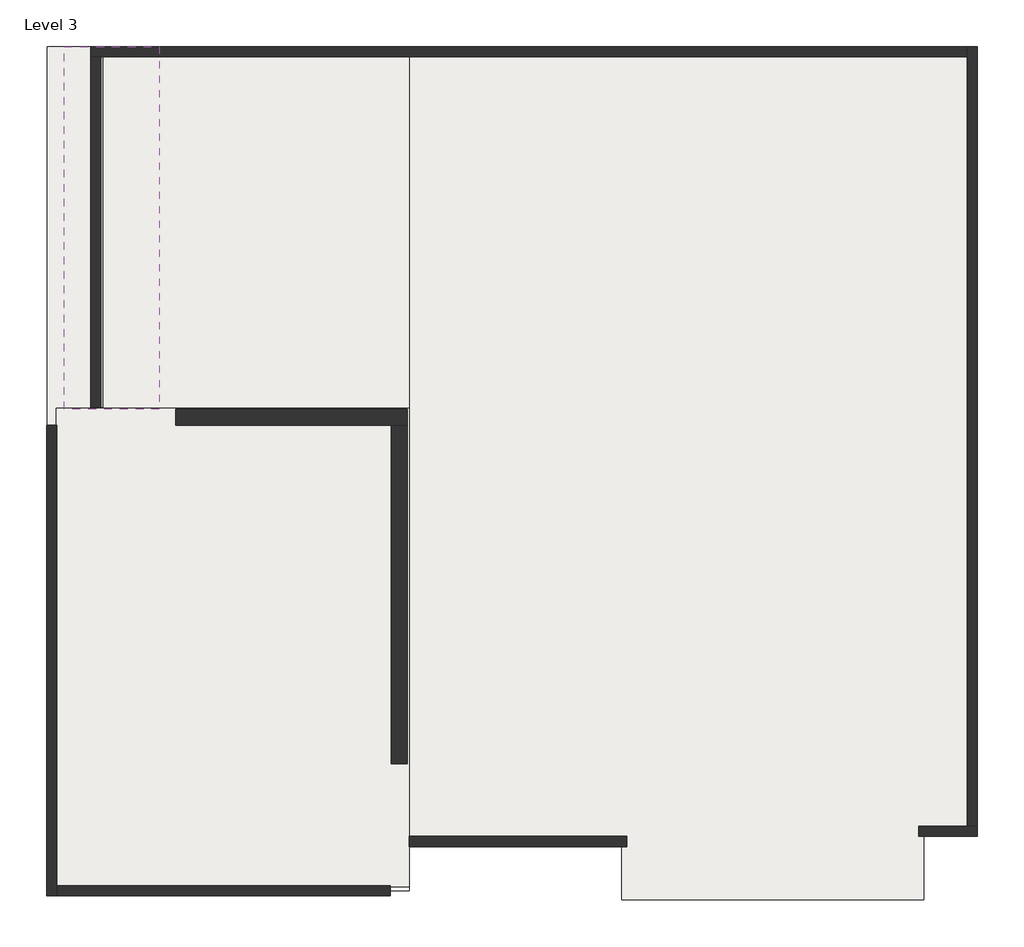
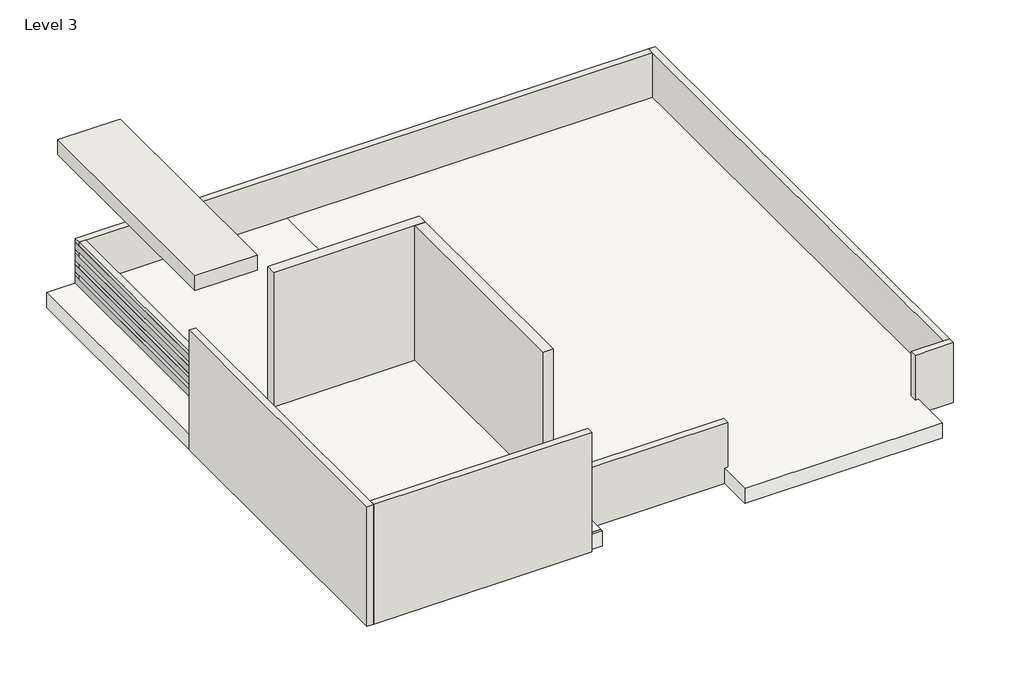
# One storey, incomplete: 10 walls, 4 proxies, 3 roofs.
"""IFC4 building model written with IfcOpenShell, lengths in millimetres."""

from ifc_helpers import new_model, si_unit, frame, origin, place, context, project, spatial, polyline, outline, extrude, faceted_brep, transform, mapped, element, save
from components import walls_6_walls_6_3012a6d8

model = new_model("IFC4")

# Units and contexts
model_context = context("Model", 3, world=origin())
ifc_project = project(units=[si_unit("LENGTHUNIT", "METRE", prefix="MILLI")], contexts=[model_context])

# Site, building, storey
site = spatial("IfcSite", under=ifc_project)
building = spatial("IfcBuilding", under=site)
storey = spatial("IfcBuildingStorey", under=building, Name="Level 3", Elevation=7315.2)

# Proxies
placement = place(None, origin())
element("IfcBuildingElementProxy", 1, Name="Reveal", ObjectType="Reveal", at=placement, inside=storey, context=model_context, shape_type="SweptSolid", body=[
    extrude(outline(polyline([(-11786.2932708, 11358.0609482), (-11633.8932708, 11358.0609482), (-11633.8932708, 6811.4609482), (-11786.2932708, 6811.4609482), (-11786.2932708, 11358.0609482)])), frame((0.0, 0.0, 8309.1450158), z_axis=(0.0, 0.0, 1.0), x_axis=(1.0, 0.0, 0.0)), (0.0, 0.0, 1.0), 152.4),
])
element("IfcBuildingElementProxy", 2, Name="Reveal", ObjectType="Reveal", at=placement, inside=storey, context=model_context, shape_type="SweptSolid", body=[
    extrude(outline(polyline([(-11786.2932708, 11358.0609482), (-11633.8932708, 11358.0609482), (-11633.8932708, 6811.4609482), (-11786.2932708, 6811.4609482), (-11786.2932708, 11358.0609482)])), frame((0.0, 0.0, 8080.5450158), z_axis=(0.0, 0.0, 1.0), x_axis=(1.0, 0.0, 0.0)), (0.0, 0.0, 1.0), 152.4),
])
element("IfcBuildingElementProxy", 3, Name="Reveal", ObjectType="Reveal", at=placement, inside=storey, context=model_context, shape_type="SweptSolid", body=[
    extrude(outline(polyline([(-11786.2932708, 11358.0609482), (-11633.8932708, 11358.0609482), (-11633.8932708, 6811.4609482), (-11786.2932708, 6811.4609482), (-11786.2932708, 11358.0609482)])), frame((0.0, 0.0, 7851.9450158), z_axis=(0.0, 0.0, 1.0), x_axis=(1.0, 0.0, 0.0)), (0.0, 0.0, 1.0), 152.4),
])
element("IfcBuildingElementProxy", 4, Name="Reveal", ObjectType="Reveal", at=placement, inside=storey, context=model_context, shape_type="SweptSolid", body=[
    extrude(outline(polyline([(-11786.2932708, 11358.0609482), (-11633.8932708, 11358.0609482), (-11633.8932708, 6811.4609482), (-11786.2932708, 6811.4609482), (-11786.2932708, 11358.0609482)])), frame((0.0, 0.0, 7620.0), z_axis=(0.0, 0.0, 1.0), x_axis=(1.0, 0.0, 0.0)), (0.0, 0.0, 1.0), 152.4),
])

# Roofs
element("IfcRoof", 5, ObjectType="Generic - 12\"", at=placement, inside=storey, context=model_context, shape_type="SweptSolid", body=[
    extrude(outline(polyline([(-11786.2932708, 11358.0609482), (-610.2932708, 11358.0609482), (-610.2932708, 1401.2609482), (-1286.2833771, 1401.2609482), (-1286.2833771, 600.2635335), (-5096.2833771, 600.2635335), (-5096.2833771, 1401.2609482), (-7773.0932708, 1401.2609482), (-7773.0932708, 1071.0609482), (-12218.0932708, 1071.0609482), (-12218.0932708, 6786.0609482), (-11786.2932708, 6786.0609482), (-11786.2932708, 11358.0609482)])), frame((0.0, 0.0, 7315.2), z_axis=(0.0, 0.0, 1.0), x_axis=(1.0, 0.0, 0.0)), (0.0, 0.0, 1.0), 304.8),
])
element("IfcRoof", 6, ObjectType="Generic - 12\"", at=placement, inside=storey, context=model_context, shape_type="SweptSolid", body=[
    extrude(outline(polyline([(-12338.7432708, 11358.0609482), (-7773.0932708, 11358.0609482), (-7773.0932708, 714.9399767), (-12338.7432708, 714.9399767), (-12338.7432708, 11358.0609482)])), frame((0.0, 0.0, 7315.2), z_axis=(0.0, 0.0, 1.0), x_axis=(1.0, 0.0, 0.0)), (0.0, 0.0, 1.0), 304.8),
])
element("IfcRoof", 7, ObjectType="Generic - 12\"", at=placement, inside=storey, context=model_context, shape_type="SweptSolid", body=[
    extrude(outline(polyline([(-7773.0932708, 765.7399767), (-12223.0431118, 765.7399767), (-12223.0431118, 6798.7609482), (-7773.0932708, 6798.7609482), (-7773.0932708, 765.7399767)])), frame((0.0, 0.0, 7315.2), z_axis=(0.0, 0.0, 1.0), x_axis=(1.0, 0.0, 0.0)), (0.0, 0.0, 1.0), 304.8),
])

# Walls
element("IfcWall", 8, ObjectType="Generic - 5\"", at=placement, inside=storey, context=model_context, shape_type="Brep", body=[
    faceted_brep([(-12345.0932708, 6582.8609482, 7315.2), (-12345.0932708, 651.9609482, 7315.2), (-12345.0932708, 651.9609482, 9753.6), (-12345.0932708, 6582.8609482, 9753.6), (-12218.0932708, 6582.8609482, 7315.2), (-12218.0932708, 6582.8609482, 9753.6), (-12218.0932708, 778.9609482, 9753.6), (-12218.0932708, 651.9609482, 9753.6), (-12218.0932708, 651.9609482, 7315.2), (-12218.0932708, 778.9609482, 7315.2)], [[[0, 1, 2, 3]], [[4, 5, 6, 7, 8, 9]], [[1, 0, 4, 9, 8]], [[3, 2, 7, 6, 5]], [[0, 3, 5, 4]], [[2, 1, 8, 7]]]),
])
element("IfcWall", 9, ObjectType="Generic - 5\"", at=placement, inside=storey, context=model_context, shape_type="SweptSolid", body=[
    extrude(outline(polyline([(-8014.3932708, 651.9609482), (-12218.0932708, 651.9609482), (-12218.0932708, 778.9609482), (-8014.3932708, 778.9609482), (-8014.3932708, 651.9609482)])), frame((0.0, 0.0, 7315.2), z_axis=(0.0, 0.0, 1.0), x_axis=(1.0, 0.0, 0.0)), (0.0, 0.0, 1.0), 2438.4),
])
element("IfcWall", 10, ObjectType="Generic - 5\"", at=placement, inside=storey, context=model_context, shape_type="Brep", body=[
    faceted_brep([(-1349.7833771, 1401.2609482, 7315.2), (-610.2932708, 1401.2609482, 7315.2), (-610.2932708, 1401.2609482, 8534.4), (-1349.7833771, 1401.2609482, 8534.4), (-1349.7833771, 1528.2609482, 7315.2), (-1349.7833771, 1528.2609482, 8534.4), (-737.2932708, 1528.2609482, 8534.4), (-610.2932708, 1528.2609482, 8534.4), (-610.2932708, 1528.2609482, 7315.2), (-737.2932708, 1528.2609482, 7315.2)], [[[0, 1, 2, 3]], [[4, 5, 6, 7, 8, 9]], [[1, 0, 4, 9, 8]], [[3, 2, 7, 6, 5]], [[0, 3, 5, 4]], [[2, 1, 8, 7]]]),
])
element("IfcWall", 11, ObjectType="Generic - 5\"", at=placement, inside=storey, context=model_context, shape_type="SweptSolid", body=[
    extrude(outline(polyline([(-7773.0932708, 1401.2609482), (-5032.7833771, 1401.2609482), (-5032.7833771, 1274.2609482), (-7773.0932708, 1274.2609482), (-7773.0932708, 1401.2609482)])), frame((0.0, 0.0, 7315.2), z_axis=(0.0, 0.0, 1.0), x_axis=(1.0, 0.0, 0.0)), (0.0, 0.0, 1.0), 1219.2),
])
element("IfcWall", 12, ObjectType="Generic - 5\"", at=placement, inside=storey, context=model_context, shape_type="Brep", body=[
    faceted_brep([(-610.2932708, 1528.2609482, 7315.2), (-610.2932708, 11358.0609482, 7315.2), (-610.2932708, 11358.0609482, 8534.4), (-610.2932708, 1528.2609482, 8534.4), (-737.2932708, 1528.2609482, 7315.2), (-737.2932708, 1528.2609482, 8534.4), (-737.2932708, 11231.0609482, 8534.4), (-737.2932708, 11358.0609482, 8534.4), (-737.2932708, 11358.0609482, 7315.2), (-737.2932708, 11231.0609482, 7315.2)], [[[0, 1, 2, 3]], [[4, 5, 6, 7, 8, 9]], [[1, 0, 4, 9, 8]], [[3, 2, 7, 6, 5]], [[0, 3, 5, 4]], [[2, 1, 8, 7]]]),
])
element("IfcWall", 13, ObjectType="Generic - 5\"", at=placement, inside=storey, context=model_context, shape_type="Brep", body=[
    faceted_brep([(-737.2932708, 11358.0609482, 7315.2), (-11786.2932708, 11358.0609482, 7315.2), (-11786.2932708, 11358.0609482, 7620.0), (-11633.8932708, 11358.0609482, 7620.0), (-11633.8932708, 11358.0609482, 7772.4), (-11786.2932708, 11358.0609482, 7772.4), (-11786.2932708, 11358.0609482, 7851.9450158), (-11633.8932708, 11358.0609482, 7851.9450158), (-11633.8932708, 11358.0609482, 8004.3450158), (-11786.2932708, 11358.0609482, 8004.3450158), (-11786.2932708, 11358.0609482, 8080.5450158), (-11633.8932708, 11358.0609482, 8080.5450158), (-11633.8932708, 11358.0609482, 8232.9450158), (-11786.2932708, 11358.0609482, 8232.9450158), (-11786.2932708, 11358.0609482, 8309.1450158), (-11633.8932708, 11358.0609482, 8309.1450158), (-11633.8932708, 11358.0609482, 8461.5450158), (-11786.2932708, 11358.0609482, 8461.5450158), (-11786.2932708, 11358.0609482, 8534.4), (-737.2932708, 11358.0609482, 8534.4), (-11786.2932708, 11231.0609482, 7315.2), (-737.2932708, 11231.0609482, 7315.2), (-737.2932708, 11231.0609482, 8534.4), (-11659.2932708, 11231.0609482, 8534.4), (-11786.2932708, 11231.0609482, 8534.4), (-11786.2932708, 11231.0609482, 8461.5450158), (-11659.2932708, 11231.0609482, 8461.5450158), (-11633.8932708, 11231.0609482, 8461.5450158), (-11633.8932708, 11231.0609482, 8309.1450158), (-11659.2932708, 11231.0609482, 8309.1450158), (-11786.2932708, 11231.0609482, 8309.1450158), (-11786.2932708, 11231.0609482, 8232.9450158), (-11659.2932708, 11231.0609482, 8232.9450158), (-11633.8932708, 11231.0609482, 8232.9450158), (-11633.8932708, 11231.0609482, 8080.5450158), (-11659.2932708, 11231.0609482, 8080.5450158), (-11786.2932708, 11231.0609482, 8080.5450158), (-11786.2932708, 11231.0609482, 8004.3450158), (-11659.2932708, 11231.0609482, 8004.3450158), (-11633.8932708, 11231.0609482, 8004.3450158), (-11633.8932708, 11231.0609482, 7851.9450158), (-11659.2932708, 11231.0609482, 7851.9450158), (-11786.2932708, 11231.0609482, 7851.9450158), (-11786.2932708, 11231.0609482, 7772.4), (-11659.2932708, 11231.0609482, 7772.4), (-11633.8932708, 11231.0609482, 7772.4), (-11633.8932708, 11231.0609482, 7620.0), (-11786.2932708, 11231.0609482, 7620.0)], [[[0, 1, 2, 3, 4, 5, 6, 7, 8, 9, 10, 11, 12, 13, 14, 15, 16, 17, 18, 19]], [[20, 21, 22, 23, 24, 25, 26, 27, 28, 29, 30, 31, 32, 33, 34, 35, 36, 37, 38, 39, 40, 41, 42, 43, 44, 45, 46, 47]], [[1, 0, 21, 20]], [[19, 18, 24, 23, 22]], [[0, 19, 22, 21]], [[1, 20, 47, 2]], [[24, 18, 17, 25]], [[30, 14, 13, 31]], [[36, 10, 9, 37]], [[42, 6, 5, 43]], [[16, 27, 26, 25, 17]], [[27, 16, 15, 28]], [[28, 15, 14, 30, 29]], [[12, 33, 32, 31, 13]], [[33, 12, 11, 34]], [[34, 11, 10, 36, 35]], [[8, 39, 38, 37, 9]], [[39, 8, 7, 40]], [[40, 7, 6, 42, 41]], [[4, 45, 44, 43, 5]], [[45, 4, 3, 46]], [[46, 3, 2, 47]]]),
])
element("IfcWall", 14, ObjectType="Generic - 5\"", at=placement, inside=storey, context=model_context, shape_type="SweptSolid", body=[
    extrude(outline(polyline([(-11786.2932708, 6811.4609482), (-11786.2932708, 11231.0609482), (-11659.2932708, 11231.0609482), (-11659.2932708, 6811.4609482), (-11786.2932708, 6811.4609482)])), frame((0.0, 0.0, 8461.5450158), z_axis=(0.0, 0.0, 1.0), x_axis=(1.0, 0.0, 0.0)), (0.0, 0.0, 1.0), 72.8549842),
    extrude(outline(polyline([(-11786.2932708, 6811.4609482), (-11786.2932708, 11231.0609482), (-11659.2932708, 11231.0609482), (-11659.2932708, 6811.4609482), (-11786.2932708, 6811.4609482)])), frame((0.0, 0.0, 8232.9450158), z_axis=(0.0, 0.0, 1.0), x_axis=(1.0, 0.0, 0.0)), (0.0, 0.0, 1.0), 76.2),
    extrude(outline(polyline([(-11786.2932708, 6811.4609482), (-11786.2932708, 11231.0609482), (-11659.2932708, 11231.0609482), (-11659.2932708, 6811.4609482), (-11786.2932708, 6811.4609482)])), frame((0.0, 0.0, 8004.3450158), z_axis=(0.0, 0.0, 1.0), x_axis=(1.0, 0.0, 0.0)), (0.0, 0.0, 1.0), 76.2),
    extrude(outline(polyline([(-11786.2932708, 6811.4609482), (-11786.2932708, 11231.0609482), (-11659.2932708, 11231.0609482), (-11659.2932708, 6811.4609482), (-11786.2932708, 6811.4609482)])), frame((0.0, 0.0, 7772.4), z_axis=(0.0, 0.0, 1.0), x_axis=(1.0, 0.0, 0.0)), (0.0, 0.0, 1.0), 79.5450158),
])
element("IfcWall", 15, ObjectType="Generic - 8\"", at=placement, inside=storey, context=model_context, shape_type="Brep", body=[
    faceted_brep([(-10719.4932708, 6582.8609482, 7315.2), (-8001.6932708, 6582.8609482, 7315.2), (-7798.4932708, 6582.8609482, 7315.2), (-7798.4932708, 6582.8609482, 10363.2), (-8001.6932708, 6582.8609482, 10363.2), (-10719.4932708, 6582.8609482, 10363.2), (-10719.4932708, 6786.0609482, 7315.2), (-10719.4932708, 6786.0609482, 10363.2), (-7798.4932708, 6786.0609482, 10363.2), (-7798.4932708, 6786.0609482, 7315.2)], [[[0, 1, 2, 3, 4, 5]], [[6, 7, 8, 9]], [[2, 1, 0, 6, 9]], [[5, 4, 3, 8, 7]], [[0, 5, 7, 6]], [[3, 2, 9, 8]]]),
])
element("IfcWall", 16, ObjectType="Generic - 8\"", at=placement, inside=storey, context=model_context, shape_type="SweptSolid", body=[
    extrude(outline(polyline([(-8001.6932708, 2315.6609482), (-8001.6932708, 6582.8609482), (-7798.4932708, 6582.8609482), (-7798.4932708, 2315.6609482), (-8001.6932708, 2315.6609482)])), frame((0.0, 0.0, 7315.2), z_axis=(0.0, 0.0, 1.0), x_axis=(1.0, 0.0, 0.0)), (0.0, 0.0, 1.0), 3048.0),
])
walls_6_walls_6_shape = walls_6_walls_6_3012a6d8(model_context)
element("IfcWall", 17, ObjectType="Walls 6 : Walls 6", at=placement, inside=storey, context=model_context, shape_type="MappedRepresentation", body=[
    mapped(walls_6_walls_6_shape, transform((0.0, 0.0, 0.0), x_axis=(1.0, 0.0, 0.0), y_axis=(0.0, 1.0, 0.0), z_axis=(0.0, 0.0, 1.0))),
])

save(model, "model.ifc")

# Revit data of these elements
# Type "Generic - 12\""
#   Assembly Code = "B1020"
#   Layers, outside or top first: 1' - 0" no material (function 1)
# Type "Generic - 5\""
#   Assembly Code = "B2010"
#   Layers, outside or top first: 0' - 5" no material (function 1)
# Type "Generic - 8\""
#   Assembly Code = "B2010"
#   Layers, outside or top first: 0' - 8" no material (function 1)
# Elements 5, 6, 7 (IfcRoof, "Generic - 12\"")
#   built-in parameter 1001705 = 25 (stored number, unit not read)
#   built-in parameter 1001710 = 33615
#   Phase Created = New Construction
#   Materials on its faces: "Default Roof"
# Elements 8, 9 (IfcWall, "Generic - 5\"")
#   Top Offset = 0' - 0"
#   Base Offset = 0' - 0"
#   Unconnected Height = 8' - 0"
#   wall height = 8' - 0"
#   Phase Created = New Construction
#   Base Constraint = Level 3
#   Materials on its faces: "Default Wall"
# Elements 10, 11, 12, 13 (IfcWall, "Generic - 5\"")
#   Top Offset = -8' - 0"
#   Base Offset = 0' - 0"
#   wall height = 4' - 0"
#   Phase Created = New Construction
#   Base Constraint = Level 3
#   Top Constraint = Level 4
#   Materials on its faces: "Default Wall"
# Element 14 (IfcWall, "Generic - 5\"")
#   built-in parameter 1001111 = 1' - 0"
#   Top Offset = -8' - 0"
#   Base Offset = 1' - 0"
#   wall height = 3' - 0"
#   Phase Created = New Construction
#   Base Constraint = Level 3
#   Top Constraint = Level 4
#   Materials on its faces: "Default Wall"
# Elements 15, 16 (IfcWall, "Generic - 8\"")
#   Top Offset = 0' - 0"
#   Base Offset = 0' - 0"
#   Unconnected Height = 10' - 0"
#   wall height = 10' - 0"
#   Phase Created = New Construction
#   Base Constraint = Level 3
#   Materials on its faces: "Default Wall"
# Element 17 (IfcWall, "Walls 6 : Walls 6")
#   Phase Created = New Construction
#   Materials on its faces: "Default Wall"
# Materials
#   "Default Roof": colour RGB 88 101 114, transparency 0
#   "Default Wall": colour RGB 128 128 128, transparency 0
